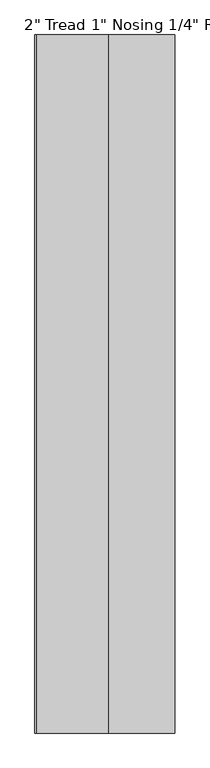
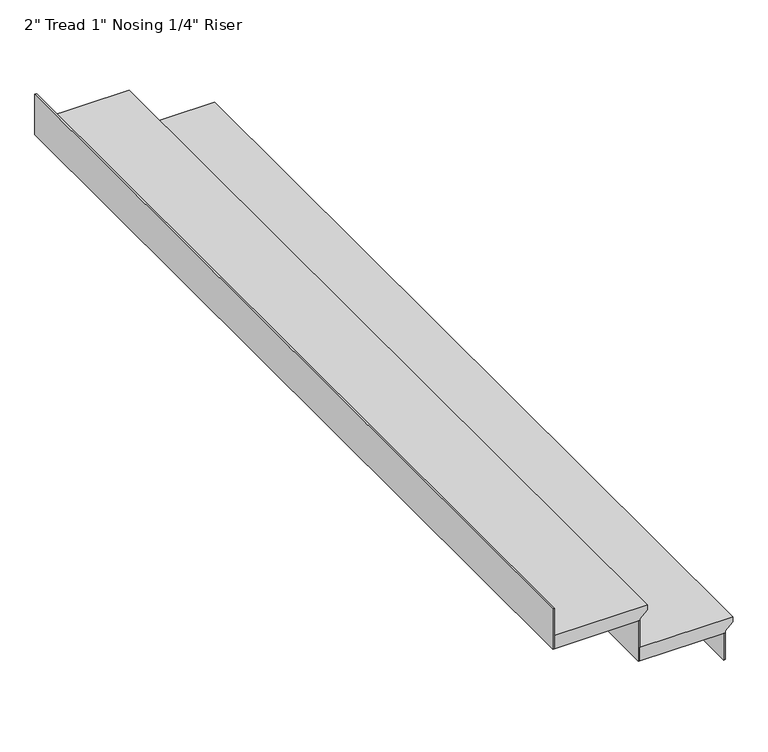
"""IFC4 building model written with IfcOpenShell, lengths in millimetres: stair flight geometry."""

from ifc_helpers import new_model, si_unit, frame, origin, origin_with_axes, place, context, project, spatial, polyline, outline, extrude, source, transform, mapped, element, save


def stair_flight_52a2f54b(model_context):
    return source(origin(), model_context, "Body", "SweptSolid", [
        extrude(outline(polyline([(152.4, -7537.7960918), (152.4, -7867.9960918), (101.6, -7867.9960918), (101.6, -7563.1960918), (107.95, -7563.1960918), (133.35, -7537.7960918), (152.4, -7537.7960918)])), frame((0.0, -11403.1453012, 0.0), z_axis=(0.0, 1.0, 0.0), x_axis=(0.0, 0.0, 1.0)), (0.0, 0.0, 1.0), 3199.3622017),
        extrude(outline(polyline([(-7569.5460918, -8203.7830995), (-7563.1960918, -8203.7830995), (-7563.1960918, -11403.1453012), (-7569.5460918, -11403.1453012), (-7569.5460918, -8203.7830995)])), origin_with_axes(), (0.0, 0.0, 1.0), 101.6),
        extrude(outline(polyline([(-7874.3460918, -8203.7830995), (-7867.9960918, -8203.7830995), (-7867.9960918, -11403.1453012), (-7874.3460918, -11403.1453012), (-7874.3460918, -8203.7830995)])), frame((0.0, 0.0, 101.6), z_axis=(0.0, 0.0, 1.0), x_axis=(1.0, 0.0, 0.0)), (0.0, 0.0, 1.0), 152.4),
        extrude(outline(polyline([(-8179.1460918, -8203.7830995), (-8172.7960918, -8203.7830995), (-8172.7960918, -11403.1453012), (-8179.1460918, -11403.1453012), (-8179.1460918, -8203.7830995)])), frame((0.0, 0.0, 254.0), z_axis=(0.0, 0.0, 1.0), x_axis=(1.0, 0.0, 0.0)), (0.0, 0.0, 1.0), 152.4),
        extrude(outline(polyline([(304.8, -7842.5960918), (304.8, -8172.7960918), (254.0, -8172.7960918), (254.0, -7867.9960918), (260.35, -7867.9960918), (285.75, -7842.5960918), (304.8, -7842.5960918)])), frame((0.0, -11403.1453012, 0.0), z_axis=(0.0, 1.0, 0.0), x_axis=(0.0, 0.0, 1.0)), (0.0, 0.0, 1.0), 3199.3622017),
    ])


if __name__ == "__main__":
    model = new_model("IFC4")
    model_context = context("Model", 3, world=origin())
    ifc_project = project(units=[si_unit("LENGTHUNIT", "METRE", prefix="MILLI")], contexts=[model_context])
    site = spatial("IfcSite", under=ifc_project)
    building = spatial("IfcBuilding", under=site)
    placement = place(None, origin())
    stair_flight_shape = stair_flight_52a2f54b(model_context)
    element("IfcStairFlight", 1, ObjectType="2\" Tread 1\" Nosing 1/4\" Riser", at=placement, inside=building, context=model_context, shape_type="MappedRepresentation", body=[
        mapped(stair_flight_shape, transform((0.0, 0.0, 0.0), x_axis=(1.0, 0.0, 0.0), y_axis=(0.0, 1.0, 0.0), z_axis=(0.0, 0.0, 1.0))),
    ])
    save(model, "model.ifc")

# Revit data of these elements
# Element 1 (IfcStairFlight, "2\" Tread 1\" Nosing 1/4\" Riser")
#   Materials on its faces: "MARBLE FLOORING 1'"
# Materials
#   "MARBLE FLOORING 1'": class "Generic", colour RGB 120 120 120, transparency 0, Cost = 0
